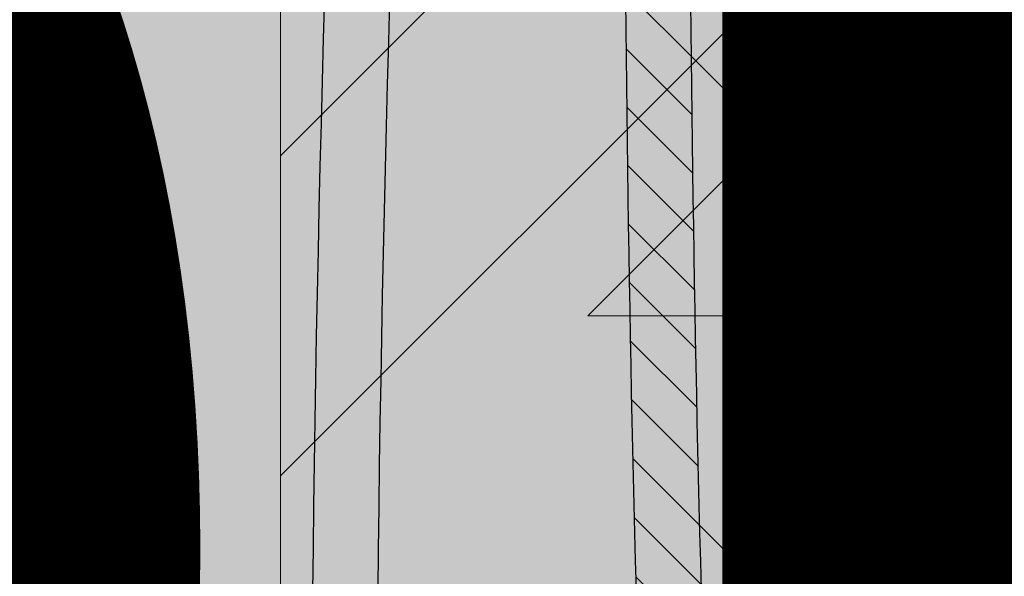
# Model space of a CAD drawing. Units: inches. Extents: x 844 to 2234, y 346 to 1084.
# Tile 76 of 93: x 1998.757 to 2001.166, y 701.365 to 702.727. Entities that reach past the tile are written whole.
import ezdxf

# ---------------------------------------------------------------- set-up
doc = ezdxf.new("R2010")
doc.units = ezdxf.units.IN
doc.header["$MEASUREMENT"] = 0
for name, color, linetype, lineweight in [('A-ANNO-DIMS', 2, 'Continuous', 18), ('furniture', 8, 'Continuous', 18), ('RA-AP-01$0$INT', 35, 'Continuous', 5)]:
    doc.layers.add(name, color=color, linetype=linetype, lineweight=lineweight)
doc.layers.add('RA-AP-01$0$FURN', color=3, linetype='Continuous')
doc.layers.add('RA-AP-01$0$WOOD', color=64, linetype='Continuous')
doc.styles.get("Standard").update_dxf_attribs({"font": 'arial.ttf'})
doc.dimstyles.get("Standard").update_dxf_attribs({"dimtxt": 6, "dimasz": 3, "dimexe": 0.18, "dimexo": 0.0625, "dimgap": 0.09, "dimtad": 0, "dimtih": 1, "dimtoh": 1, "dimdec": 1, "dimzin": 0, "dimdsep": 46, "dimlunit": 3, "dimtxsty": 'Standard', "dimblk": 'ARCHTICK', "dimcen": 0.09, "dimadec": 0, "dimazin": 0, "dimtfac": 1, "dimtdec": 1, "dimtofl": 0, "dimtmove": 0, "dimatfit": 3, "dimfxl": 1, "dimtolj": 1, "dimtzin": 0, "dimarcsym": 0})

# ---------------------------------------------------------------- blocks, each defined once
blk = doc.blocks.new('A$C18D01794')
at = {"layer": 'RA-AP-01$0$INT'}
h = blk.add_hatch(color=256, dxfattribs=at)
h.paths.add_polyline_path([(4.46935, -7.07085), (4.50521, -7.035), (4.50521, -7.10671)])
h.paths.add_polyline_path([(4.45521, -7.085), (4.47692, -7.10671), (4.43349, -7.10671)])
h.paths.add_polyline_path([(4.40521, -7.035), (4.44106, -7.07085), (4.40521, -7.10671)])
h.paths.add_polyline_path([(4.42521, -6.91146), (4.45521, -6.88146), (4.48521, -6.91146), (4.48521, -7.02671), (4.45521, -7.05671), (4.42521, -7.02671)])
h.paths.add_polyline_path([(4.50521, -6.83146), (4.50521, -6.90318), (4.46935, -6.86732)])
h.paths.add_polyline_path([(4.42521, -6.70793), (4.45521, -6.67793), (4.48521, -6.70793), (4.48521, -6.82318), (4.45521, -6.85318), (4.42521, -6.82318)])
h.paths.add_polyline_path([(4.42521, -6.50439), (4.45521, -6.47439), (4.48521, -6.50439), (4.48521, -6.61964), (4.45521, -6.64964), (4.42521, -6.61964)])
h.paths.add_polyline_path([(4.46935, -6.66378), (4.50521, -6.62793), (4.50521, -6.69964)])
h.paths.add_polyline_path([(4.40521, -6.62793), (4.44106, -6.66378), (4.40521, -6.69964)])
h.paths.add_polyline_path([(4.40521, -6.42439), (4.44106, -6.46025), (4.40521, -6.49611)])
h.paths.add_polyline_path([(4.46935, -6.46025), (4.50521, -6.42439), (4.50521, -6.49611)])
h.paths.add_polyline_path([(4.42521, -6.30085), (4.45521, -6.27085), (4.48521, -6.30085), (4.48521, -6.41611), (4.45521, -6.44611), (4.42521, -6.41611)])
h.paths.add_polyline_path([(4.42521, -6.22671), (4.47106, -6.22671), (4.42521, -6.27257)])
h.paths.add_polyline_path([(4.49935, -6.22671), (4.63606, -6.22671), (4.66606, -6.25671), (4.63606, -6.28671), (4.49935, -6.28671), (4.46935, -6.25671)])
h.paths.add_polyline_path([(4.68021, -6.27085), (4.71606, -6.30671), (4.64435, -6.30671)])
h.paths.add_polyline_path([(4.64435, -6.20671), (4.71606, -6.20671), (4.68021, -6.24257)])
h.paths.add_polyline_path([(4.72435, -6.22671), (4.86106, -6.22671), (4.89106, -6.25671), (4.86106, -6.28671), (4.72435, -6.28671), (4.69435, -6.25671)])
h.paths.add_polyline_path([(4.90521, -6.27085), (4.94106, -6.30671), (4.86935, -6.30671)])
h.paths.add_polyline_path([(4.86935, -6.20671), (4.94106, -6.20671), (4.90521, -6.24257)])
h.paths.add_polyline_path([(4.94935, -6.22671), (5.08606, -6.22671), (5.11606, -6.25671), (5.08606, -6.28671), (4.94935, -6.28671), (4.91935, -6.25671)])
h.paths.add_polyline_path([(5.13021, -6.27085), (5.16606, -6.30671), (5.09435, -6.30671)])
h.paths.add_polyline_path([(5.09435, -6.20671), (5.16606, -6.20671), (5.13021, -6.24257)])
h.paths.add_polyline_path([(5.17435, -6.22671), (5.31106, -6.22671), (5.34106, -6.25671), (5.31106, -6.28671), (5.17435, -6.28671), (5.14435, -6.25671)])
h.paths.add_polyline_path([(5.32521, -6.30085), (5.35521, -6.27085), (5.38521, -6.30085), (5.38521, -6.41611), (5.35521, -6.44611), (5.32521, -6.41611)])
h.paths.add_polyline_path([(5.33935, -6.22671), (5.38521, -6.22671), (5.38521, -6.27257)])
h.paths.add_polyline_path([(5.32521, -6.50439), (5.35521, -6.47439), (5.38521, -6.50439), (5.38521, -6.61964), (5.35521, -6.64964), (5.32521, -6.61964)])
h.paths.add_polyline_path([(5.30521, -6.42439), (5.34106, -6.46025), (5.30521, -6.49611)])
h.paths.add_polyline_path([(5.36935, -6.46025), (5.40521, -6.42439), (5.40521, -6.49611)])
h.paths.add_polyline_path([(5.40521, -6.62793), (5.40521, -6.69964), (5.36935, -6.66378)])
h.paths.add_polyline_path([(5.30521, -6.62793), (5.34106, -6.66378), (5.30521, -6.69964)])
h.paths.add_polyline_path([(5.32521, -6.70793), (5.35521, -6.67793), (5.38521, -6.70793), (5.38521, -6.82318), (5.35521, -6.85318), (5.32521, -6.82318)])
h.paths.add_polyline_path([(5.30521, -6.83146), (5.34106, -6.86732), (5.30521, -6.90318)])
h.paths.add_polyline_path([(5.32521, -6.91146), (5.35521, -6.88146), (5.38521, -6.91146), (5.38521, -7.02671), (5.35521, -7.05671), (5.32521, -7.02671)])
h.paths.add_polyline_path([(5.40458, -6.83209, 0.001218), (5.40521, -6.83231), (5.40521, -6.90318), (5.36935, -6.86732)])
h.paths.add_polyline_path([(5.36935, -7.07085), (5.40521, -7.035), (5.40521, -7.10671)])
h.paths.add_polyline_path([(5.35521, -7.085), (5.37692, -7.10671), (5.33349, -7.10671)])
h.paths.add_polyline_path([(5.30521, -7.035), (5.34106, -7.07085), (5.30521, -7.10671)])
for points in [[(4.50521, -6.30671), (5.30521, -6.30671), (5.30521, -7.10671), (5.25521, -7.10671), (5.25521, -6.35671), (4.55521, -6.35671), (4.55521, -7.10671), (4.50521, -7.10671)], [(4.50521, -7.90671), (5.30521, -7.90671), (5.30521, -7.10671), (5.25521, -7.10671), (5.25521, -7.85671), (4.55521, -7.85671), (4.55521, -7.10671), (4.50521, -7.10671)]]:
    blk.add_hatch(color=256, dxfattribs=at).paths.add_polyline_path(points)
h = blk.add_hatch(color=256, dxfattribs=at)
h.paths.add_polyline_path([(4.58592, -6.35671), (4.6142, -6.35671), (4.66885, -6.41136), (4.72349, -6.35671), (4.77177, -6.35671), (4.82642, -6.41136), (4.86278, -6.375), (4.8445, -6.35671), (4.86278, -6.35671), (4.90521, -6.39914), (4.94763, -6.35671), (4.96592, -6.35671), (4.94763, -6.375), (4.98399, -6.41136), (5.03864, -6.35671), (5.08692, -6.35671), (5.14157, -6.41136), (5.19621, -6.35671), (5.2245, -6.35671), (4.90521, -6.676)])
h.paths.add_polyline_path([(4.89521, -6.63772), (4.89521, -6.52843), (4.84056, -6.58307)], flags=16)
h.paths.add_polyline_path([(4.91521, -6.63772), (4.96985, -6.58307), (4.91521, -6.52843)], flags=16)
h.paths.add_polyline_path([(4.82642, -6.56893), (4.88106, -6.51429), (4.77177, -6.51429)], flags=16)
h.paths.add_polyline_path([(4.98399, -6.56893), (5.03864, -6.51429), (4.92935, -6.51429)], flags=16)
h.paths.add_polyline_path([(4.88106, -6.49429), (4.82642, -6.43964), (4.77177, -6.49429)], flags=16)
h.paths.add_polyline_path([(4.92935, -6.49429), (5.03864, -6.49429), (4.98399, -6.43964)], flags=16)
h.paths.add_polyline_path([(4.89521, -6.48014), (4.89521, -6.40742), (4.87692, -6.38914), (4.84056, -6.4255)], flags=16)
h.paths.add_polyline_path([(4.91521, -6.48014), (4.96985, -6.4255), (4.93349, -6.38914), (4.91521, -6.40742)], flags=16)
h.paths.add_polyline_path([(4.75763, -6.48014), (4.81228, -6.4255), (4.75763, -6.37085)], flags=16)
h.paths.add_polyline_path([(4.73763, -6.48014), (4.73763, -6.37085), (4.68299, -6.4255)], flags=16)
h.paths.add_polyline_path([(5.05278, -6.48014), (5.05278, -6.37085), (4.99814, -6.4255)], flags=16)
h.paths.add_polyline_path([(5.07278, -6.48014), (5.12742, -6.4255), (5.07278, -6.37085)], flags=16)
h.paths.add_polyline_path([(4.93592, -6.70671), (5.25521, -6.38742), (5.25521, -6.41571), (5.20056, -6.47035), (5.25521, -6.525), (5.25521, -6.57328), (5.20056, -6.62793), (5.23692, -6.66429), (5.25521, -6.646), (5.25521, -6.66429), (5.21278, -6.70671), (5.25521, -6.74914), (5.25521, -6.76742), (5.23692, -6.74914), (5.20056, -6.7855), (5.25521, -6.84014), (5.25521, -6.88843), (5.20056, -6.94307), (5.25521, -6.99772), (5.25521, -7.026)])
h.paths.add_polyline_path([(5.04299, -6.7855), (5.09763, -6.84014), (5.09763, -6.73085)], flags=16)
h.paths.add_polyline_path([(5.02885, -6.77136), (5.08349, -6.71671), (4.9742, -6.71671)], flags=16)
h.paths.add_polyline_path([(5.11763, -6.84014), (5.17228, -6.7855), (5.11763, -6.73085)], flags=16)
h.paths.add_polyline_path([(5.08349, -6.69671), (5.02885, -6.64207), (4.9742, -6.69671)], flags=16)
h.paths.add_polyline_path([(5.13177, -6.85429), (5.18642, -6.79964), (5.24106, -6.85429)], flags=17)
h.paths.add_polyline_path([(5.13177, -6.71671), (5.18642, -6.77136), (5.22278, -6.735), (5.2045, -6.71671)], flags=16)
h.paths.add_polyline_path([(5.09763, -6.68257), (5.09763, -6.57328), (5.04299, -6.62793)], flags=16)
h.paths.add_polyline_path([(5.13177, -6.87429), (5.24106, -6.87429), (5.18642, -6.92893)], flags=17)
h.paths.add_polyline_path([(5.13177, -6.69671), (5.2045, -6.69671), (5.22278, -6.67843), (5.18642, -6.64207)], flags=16)
h.paths.add_polyline_path([(5.11763, -6.68257), (5.17228, -6.62793), (5.11763, -6.57328)], flags=16)
h.paths.add_polyline_path([(5.18642, -6.61378), (5.24106, -6.55914), (5.13177, -6.55914)], flags=16)
h.paths.add_polyline_path([(5.13177, -6.53914), (5.24106, -6.53914), (5.18642, -6.48449)], flags=16)
h.paths.add_polyline_path([(5.25521, -7.08742), (5.25521, -7.10671), (4.55521, -7.10671), (4.55521, -7.08742), (4.90521, -6.73742)])
h.paths.add_polyline_path([(4.98399, -6.84449), (4.92935, -6.89914), (5.03864, -6.89914)], flags=16)
h.paths.add_polyline_path([(4.96985, -6.83035), (4.91521, -6.77571), (4.91521, -6.885)], flags=16)
h.paths.add_polyline_path([(4.92935, -6.91914), (4.98399, -6.97378), (5.03864, -6.91914)], flags=16)
h.paths.add_polyline_path([(5.05278, -6.93328), (4.99814, -6.98793), (5.05278, -7.04257)], flags=16)
h.paths.add_polyline_path([(5.07278, -6.93328), (5.07278, -7.04257), (5.12742, -6.98793)], flags=16)
h.paths.add_polyline_path([(4.89521, -6.77571), (4.84056, -6.83035), (4.89521, -6.885)], flags=16)
h.paths.add_polyline_path([(4.91521, -6.93328), (4.91521, -7.006), (4.93349, -7.02429), (4.96985, -6.98793)], flags=16)
h.paths.add_polyline_path([(4.88106, -6.89914), (4.82642, -6.84449), (4.77177, -6.89914)], flags=16)
h.paths.add_polyline_path([(4.89521, -6.93328), (4.84056, -6.98793), (4.87692, -7.02429), (4.89521, -7.006)], flags=16)
h.paths.add_polyline_path([(4.98399, -7.00207), (4.94763, -7.03843), (4.96592, -7.05671), (5.03864, -7.05671)], flags=16)
h.paths.add_polyline_path([(4.88106, -6.91914), (4.77177, -6.91914), (4.82642, -6.97378)], flags=16)
h.paths.add_polyline_path([(4.90521, -7.01429), (4.86278, -7.05671), (4.94763, -7.05671)], flags=16)
h.paths.add_polyline_path([(5.14157, -7.00207), (5.08692, -7.05671), (5.19621, -7.05671)], flags=16)
h.paths.add_polyline_path([(4.82642, -7.00207), (4.77177, -7.05671), (4.8445, -7.05671), (4.86278, -7.03843)], flags=16)
h.paths.add_polyline_path([(4.81228, -6.98793), (4.75763, -6.93328), (4.75763, -7.04257)], flags=16)
h.paths.add_polyline_path([(4.73763, -6.93328), (4.68299, -6.98793), (4.73763, -7.04257)], flags=16)
h.paths.add_polyline_path([(4.72349, -7.05671), (4.66885, -7.00207), (4.6142, -7.05671)], flags=16)
h.paths.add_polyline_path([(4.59763, -6.70671), (4.55521, -6.66429), (4.55521, -6.646), (4.57349, -6.66429), (4.60985, -6.62793), (4.55521, -6.57328), (4.55521, -6.525), (4.60985, -6.47035), (4.55521, -6.41571), (4.55521, -6.38742), (4.8745, -6.70671), (4.55521, -7.026), (4.55521, -6.99772), (4.60985, -6.94307), (4.55521, -6.88843), (4.55521, -6.84014), (4.60985, -6.7855), (4.57349, -6.74914), (4.55521, -6.76742), (4.55521, -6.74914)])
h.paths.add_polyline_path([(4.71278, -6.73085), (4.71278, -6.84014), (4.76742, -6.7855)], flags=16)
h.paths.add_polyline_path([(4.72692, -6.71671), (4.78157, -6.77136), (4.83621, -6.71671)], flags=16)
h.paths.add_polyline_path([(4.69278, -6.73085), (4.63814, -6.7855), (4.69278, -6.84014)], flags=16)
h.paths.add_polyline_path([(4.72692, -6.69671), (4.83621, -6.69671), (4.78157, -6.64207)], flags=16)
h.paths.add_polyline_path([(4.67864, -6.71671), (4.60592, -6.71671), (4.58763, -6.735), (4.62399, -6.77136)], flags=16)
h.paths.add_polyline_path([(4.71278, -6.68257), (4.76742, -6.62793), (4.71278, -6.57328)], flags=16)
h.paths.add_polyline_path([(4.67864, -6.69671), (4.62399, -6.64207), (4.58763, -6.67843), (4.60592, -6.69671)], flags=16)
h.paths.add_polyline_path([(4.69278, -6.68257), (4.69278, -6.57328), (4.63814, -6.62793)], flags=16)
h.paths.add_polyline_path([(4.62399, -6.79964), (4.67864, -6.85429), (4.56935, -6.85429)], flags=17)
h.paths.add_polyline_path([(4.62399, -6.61378), (4.67864, -6.55914), (4.56935, -6.55914)], flags=16)
h.paths.add_polyline_path([(4.67864, -6.87429), (4.62399, -6.92893), (4.56935, -6.87429)], flags=17)
h.paths.add_polyline_path([(4.67864, -6.53914), (4.62399, -6.48449), (4.56935, -6.53914)], flags=16)
h = blk.add_hatch(color=256, dxfattribs=at)
h.paths.add_polyline_path([(4.50521, -7.5855), (4.46935, -7.54964), (4.50521, -7.51378), (4.50521, -7.38196), (4.46935, -7.34611), (4.50521, -7.31025), (4.50521, -7.17843), (4.46935, -7.14257), (4.50521, -7.10671), (4.47692, -7.10671), (4.45521, -7.12843), (4.43349, -7.10671), (4.40521, -7.10671), (4.44106, -7.14257), (4.40521, -7.17843), (4.40521, -7.31025), (4.44106, -7.34611), (4.40521, -7.38196), (4.40521, -7.51378), (4.44106, -7.54964), (4.40521, -7.5855), (4.40521, -7.71732), (4.44106, -7.75318), (4.40521, -7.78903), (4.40521, -8.00671), (4.64435, -8.00671), (4.68021, -7.97085), (4.71606, -8.00671), (4.86935, -8.00671), (4.90521, -7.97085), (4.94106, -8.00671), (5.09435, -8.00671), (5.13021, -7.97085), (5.16606, -8.00671), (5.40521, -8.00671), (5.40521, -7.78903), (5.36935, -7.75318), (5.40521, -7.71732), (5.40521, -7.5855), (5.36935, -7.54964), (5.40521, -7.51378), (5.40521, -7.38196), (5.36935, -7.34611), (5.40521, -7.31025), (5.40521, -7.17843), (5.36935, -7.14257), (5.40521, -7.10671), (5.37692, -7.10671), (5.35521, -7.12843), (5.33349, -7.10671), (5.30521, -7.10671), (5.34106, -7.14257), (5.30521, -7.17843), (5.30521, -7.31025), (5.34106, -7.34611), (5.30521, -7.38196), (5.30521, -7.51378), (5.34106, -7.54964), (5.30521, -7.5855), (5.30521, -7.71732), (5.34106, -7.75318), (5.30521, -7.78903), (5.30521, -7.90671), (5.16606, -7.90671), (5.13021, -7.94257), (5.09435, -7.90671), (4.94106, -7.90671), (4.90521, -7.94257), (4.86935, -7.90671), (4.71606, -7.90671), (4.68021, -7.94257), (4.64435, -7.90671), (4.50521, -7.90671), (4.50521, -7.78903), (4.46935, -7.75318), (4.50521, -7.71732)])
h.paths.add_polyline_path([(4.48521, -7.70903), (4.45521, -7.73903), (4.42521, -7.70903), (4.42521, -7.59378), (4.45521, -7.56378), (4.48521, -7.59378)], flags=16)
h.paths.add_polyline_path([(4.45521, -7.76732), (4.48521, -7.79732), (4.48521, -7.91257), (4.45521, -7.94257), (4.42521, -7.91257), (4.42521, -7.79732)], flags=16)
h.paths.add_polyline_path([(4.45521, -7.5355), (4.42521, -7.5055), (4.42521, -7.39025), (4.45521, -7.36025), (4.48521, -7.39025), (4.48521, -7.5055)], flags=16)
h.paths.add_polyline_path([(4.49935, -7.92671), (4.63606, -7.92671), (4.66606, -7.95671), (4.63606, -7.98671), (4.49935, -7.98671), (4.46935, -7.95671)], flags=16)
h.paths.add_polyline_path([(4.42521, -7.94085), (4.47106, -7.98671), (4.42521, -7.98671)], flags=16)
h.paths.add_polyline_path([(4.45521, -7.33196), (4.42521, -7.30196), (4.42521, -7.18671), (4.45521, -7.15671), (4.48521, -7.18671), (4.48521, -7.30196)], flags=16)
h.paths.add_polyline_path([(4.72435, -7.92671), (4.86106, -7.92671), (4.89106, -7.95671), (4.86106, -7.98671), (4.72435, -7.98671), (4.69435, -7.95671)], flags=16)
h.paths.add_polyline_path([(4.91935, -7.95671), (4.94935, -7.92671), (5.08606, -7.92671), (5.11606, -7.95671), (5.08606, -7.98671), (4.94935, -7.98671)], flags=16)
h.paths.add_polyline_path([(5.14435, -7.95671), (5.17435, -7.92671), (5.31106, -7.92671), (5.34106, -7.95671), (5.31106, -7.98671), (5.17435, -7.98671)], flags=16)
h.paths.add_polyline_path([(5.32521, -7.59378), (5.35521, -7.56378), (5.38521, -7.59378), (5.38521, -7.70903), (5.35521, -7.73903), (5.32521, -7.70903)], flags=16)
h.paths.add_polyline_path([(5.32521, -7.79732), (5.35521, -7.76732), (5.38521, -7.79732), (5.38521, -7.91257), (5.35521, -7.94257), (5.32521, -7.91257)], flags=16)
h.paths.add_polyline_path([(5.32521, -7.5055), (5.32521, -7.39025), (5.35521, -7.36025), (5.38521, -7.39025), (5.38521, -7.5055), (5.35521, -7.5355)], flags=16)
h.paths.add_polyline_path([(5.32521, -7.30196), (5.32521, -7.18671), (5.35521, -7.15671), (5.38521, -7.18671), (5.38521, -7.30196), (5.35521, -7.33196)], flags=16)
h.paths.add_polyline_path([(5.33935, -7.98671), (5.38521, -7.94085), (5.38521, -7.98671)], flags=16)
h = blk.add_hatch(color=256, dxfattribs=at)
h.paths.add_polyline_path([(4.46935, -7.14257), (4.50521, -7.17843), (4.50521, -7.10671)])
h.paths.add_polyline_path([(4.45521, -7.12843), (4.47692, -7.10671), (4.43349, -7.10671)])
h.paths.add_polyline_path([(4.40521, -7.17843), (4.44106, -7.14257), (4.40521, -7.10671)])
h.paths.add_polyline_path([(4.42521, -7.30196), (4.45521, -7.33196), (4.48521, -7.30196), (4.48521, -7.18671), (4.45521, -7.15671), (4.42521, -7.18671)])
h.paths.add_polyline_path([(4.50521, -7.38196), (4.50521, -7.31025), (4.46935, -7.34611)])
h.paths.add_polyline_path([(4.42521, -7.5055), (4.45521, -7.5355), (4.48521, -7.5055), (4.48521, -7.39025), (4.45521, -7.36025), (4.42521, -7.39025)])
h.paths.add_polyline_path([(4.42521, -7.70903), (4.45521, -7.73903), (4.48521, -7.70903), (4.48521, -7.59378), (4.45521, -7.56378), (4.42521, -7.59378)])
h.paths.add_polyline_path([(4.46935, -7.54964), (4.50521, -7.5855), (4.50521, -7.51378)])
h.paths.add_polyline_path([(4.40521, -7.5855), (4.44106, -7.54964), (4.40521, -7.51378)])
h.paths.add_polyline_path([(4.40521, -7.78903), (4.44106, -7.75318), (4.40521, -7.71732)])
h.paths.add_polyline_path([(4.46935, -7.75318), (4.50521, -7.78903), (4.50521, -7.71732)])
h.paths.add_polyline_path([(4.42521, -7.91257), (4.45521, -7.94257), (4.48521, -7.91257), (4.48521, -7.79732), (4.45521, -7.76732), (4.42521, -7.79732)])
h.paths.add_polyline_path([(4.42521, -7.98671), (4.47106, -7.98671), (4.42521, -7.94085)])
h.paths.add_polyline_path([(4.49935, -7.98671), (4.63606, -7.98671), (4.66606, -7.95671), (4.63606, -7.92671), (4.49935, -7.92671), (4.46935, -7.95671)])
h.paths.add_polyline_path([(4.68021, -7.94257), (4.71606, -7.90671), (4.64435, -7.90671)])
h.paths.add_polyline_path([(4.64435, -8.00671), (4.71606, -8.00671), (4.68021, -7.97085)])
h.paths.add_polyline_path([(4.72435, -7.98671), (4.86106, -7.98671), (4.89106, -7.95671), (4.86106, -7.92671), (4.72435, -7.92671), (4.69435, -7.95671)])
h.paths.add_polyline_path([(4.90521, -7.94257), (4.94106, -7.90671), (4.86935, -7.90671)])
h.paths.add_polyline_path([(4.86935, -8.00671), (4.94106, -8.00671), (4.90521, -7.97085)])
h.paths.add_polyline_path([(4.94935, -7.98671), (5.08606, -7.98671), (5.11606, -7.95671), (5.08606, -7.92671), (4.94935, -7.92671), (4.91935, -7.95671)])
h.paths.add_polyline_path([(5.13021, -7.94257), (5.16606, -7.90671), (5.09435, -7.90671)])
h.paths.add_polyline_path([(5.09435, -8.00671), (5.16606, -8.00671), (5.13021, -7.97085)])
h.paths.add_polyline_path([(5.17435, -7.98671), (5.31106, -7.98671), (5.34106, -7.95671), (5.31106, -7.92671), (5.17435, -7.92671), (5.14435, -7.95671)])
h.paths.add_polyline_path([(5.32521, -7.91257), (5.35521, -7.94257), (5.38521, -7.91257), (5.38521, -7.79732), (5.35521, -7.76732), (5.32521, -7.79732)])
h.paths.add_polyline_path([(5.33935, -7.98671), (5.38521, -7.98671), (5.38521, -7.94085)])
h.paths.add_polyline_path([(5.32521, -7.70903), (5.35521, -7.73903), (5.38521, -7.70903), (5.38521, -7.59378), (5.35521, -7.56378), (5.32521, -7.59378)])
h.paths.add_polyline_path([(5.30521, -7.78903), (5.34106, -7.75318), (5.30521, -7.71732)])
h.paths.add_polyline_path([(5.36935, -7.75318), (5.40521, -7.78903), (5.40521, -7.71732)])
h.paths.add_polyline_path([(5.40521, -7.5855), (5.40521, -7.51378), (5.36935, -7.54964)])
h.paths.add_polyline_path([(5.30521, -7.5855), (5.34106, -7.54964), (5.30521, -7.51378)])
h.paths.add_polyline_path([(5.32521, -7.5055), (5.35521, -7.5355), (5.38521, -7.5055), (5.38521, -7.39025), (5.35521, -7.36025), (5.32521, -7.39025)])
h.paths.add_polyline_path([(5.30521, -7.38196), (5.34106, -7.34611), (5.30521, -7.31025)])
h.paths.add_polyline_path([(5.32521, -7.30196), (5.35521, -7.33196), (5.38521, -7.30196), (5.38521, -7.18671), (5.35521, -7.15671), (5.32521, -7.18671)])
h.paths.add_polyline_path([(5.40458, -7.38134, -0.001218), (5.40521, -7.38111), (5.40521, -7.31025), (5.36935, -7.34611)])
h.paths.add_polyline_path([(5.36935, -7.14257), (5.40521, -7.17843), (5.40521, -7.10671)])
h.paths.add_polyline_path([(5.35521, -7.12843), (5.37692, -7.10671), (5.33349, -7.10671)])
h.paths.add_polyline_path([(5.30521, -7.17843), (5.34106, -7.14257), (5.30521, -7.10671)])
h = blk.add_hatch(color=256, dxfattribs=at)
h.paths.add_polyline_path([(4.58592, -7.85671), (4.6142, -7.85671), (4.66885, -7.80207), (4.72349, -7.85671), (4.77177, -7.85671), (4.82642, -7.80207), (4.86278, -7.83843), (4.8445, -7.85671), (4.86278, -7.85671), (4.90521, -7.81429), (4.94763, -7.85671), (4.96592, -7.85671), (4.94763, -7.83843), (4.98399, -7.80207), (5.03864, -7.85671), (5.08692, -7.85671), (5.14157, -7.80207), (5.19621, -7.85671), (5.2245, -7.85671), (4.90521, -7.53742)])
h.paths.add_polyline_path([(4.89521, -7.57571), (4.89521, -7.685), (4.84056, -7.63035)], flags=16)
h.paths.add_polyline_path([(4.91521, -7.57571), (4.96985, -7.63035), (4.91521, -7.685)], flags=16)
h.paths.add_polyline_path([(4.82642, -7.64449), (4.88106, -7.69914), (4.77177, -7.69914)], flags=16)
h.paths.add_polyline_path([(4.98399, -7.64449), (5.03864, -7.69914), (4.92935, -7.69914)], flags=16)
h.paths.add_polyline_path([(4.88106, -7.71914), (4.82642, -7.77378), (4.77177, -7.71914)], flags=16)
h.paths.add_polyline_path([(4.92935, -7.71914), (5.03864, -7.71914), (4.98399, -7.77378)], flags=16)
h.paths.add_polyline_path([(4.89521, -7.73328), (4.89521, -7.806), (4.87692, -7.82429), (4.84056, -7.78793)], flags=16)
h.paths.add_polyline_path([(4.91521, -7.73328), (4.96985, -7.78793), (4.93349, -7.82429), (4.91521, -7.806)], flags=16)
h.paths.add_polyline_path([(4.75763, -7.73328), (4.81228, -7.78793), (4.75763, -7.84257)], flags=16)
h.paths.add_polyline_path([(4.73763, -7.73328), (4.73763, -7.84257), (4.68299, -7.78793)], flags=16)
h.paths.add_polyline_path([(5.05278, -7.73328), (5.05278, -7.84257), (4.99814, -7.78793)], flags=16)
h.paths.add_polyline_path([(5.07278, -7.73328), (5.12742, -7.78793), (5.07278, -7.84257)], flags=16)
h.paths.add_polyline_path([(4.93592, -7.50671), (5.25521, -7.826), (5.25521, -7.79772), (5.20056, -7.74307), (5.25521, -7.68843), (5.25521, -7.64014), (5.20056, -7.5855), (5.23692, -7.54914), (5.25521, -7.56742), (5.25521, -7.54914), (5.21278, -7.50671), (5.25521, -7.46429), (5.25521, -7.446), (5.23692, -7.46429), (5.20056, -7.42793), (5.25521, -7.37328), (5.25521, -7.325), (5.20056, -7.27035), (5.25521, -7.21571), (5.25521, -7.18742)])
h.paths.add_polyline_path([(5.04299, -7.42793), (5.09763, -7.37328), (5.09763, -7.48257)], flags=16)
h.paths.add_polyline_path([(5.02885, -7.44207), (5.08349, -7.49671), (4.9742, -7.49671)], flags=16)
h.paths.add_polyline_path([(5.11763, -7.37328), (5.17228, -7.42793), (5.11763, -7.48257)], flags=16)
h.paths.add_polyline_path([(5.08349, -7.51671), (5.02885, -7.57136), (4.9742, -7.51671)], flags=16)
h.paths.add_polyline_path([(5.13177, -7.35914), (5.18642, -7.41378), (5.24106, -7.35914)], flags=17)
h.paths.add_polyline_path([(5.13177, -7.49671), (5.18642, -7.44207), (5.22278, -7.47843), (5.2045, -7.49671)], flags=16)
h.paths.add_polyline_path([(5.09763, -7.53085), (5.09763, -7.64014), (5.04299, -7.5855)], flags=16)
h.paths.add_polyline_path([(5.13177, -7.33914), (5.24106, -7.33914), (5.18642, -7.28449)], flags=17)
h.paths.add_polyline_path([(5.13177, -7.51671), (5.2045, -7.51671), (5.22278, -7.535), (5.18642, -7.57136)], flags=16)
h.paths.add_polyline_path([(5.11763, -7.53085), (5.17228, -7.5855), (5.11763, -7.64014)], flags=16)
h.paths.add_polyline_path([(5.18642, -7.59964), (5.24106, -7.65429), (5.13177, -7.65429)], flags=16)
h.paths.add_polyline_path([(5.13177, -7.67429), (5.24106, -7.67429), (5.18642, -7.72893)], flags=16)
h.paths.add_polyline_path([(5.25521, -7.126), (5.25521, -7.10671), (4.55521, -7.10671), (4.55521, -7.126), (4.90521, -7.476)])
h.paths.add_polyline_path([(4.98399, -7.36893), (4.92935, -7.31429), (5.03864, -7.31429)], flags=16)
h.paths.add_polyline_path([(4.96985, -7.38307), (4.91521, -7.43772), (4.91521, -7.32843)], flags=16)
h.paths.add_polyline_path([(4.92935, -7.29429), (4.98399, -7.23964), (5.03864, -7.29429)], flags=16)
h.paths.add_polyline_path([(5.05278, -7.28014), (4.99814, -7.2255), (5.05278, -7.17085)], flags=16)
h.paths.add_polyline_path([(5.07278, -7.28014), (5.07278, -7.17085), (5.12742, -7.2255)], flags=16)
h.paths.add_polyline_path([(4.89521, -7.43772), (4.84056, -7.38307), (4.89521, -7.32843)], flags=16)
h.paths.add_polyline_path([(4.91521, -7.28014), (4.91521, -7.20742), (4.93349, -7.18914), (4.96985, -7.2255)], flags=16)
h.paths.add_polyline_path([(4.88106, -7.31429), (4.82642, -7.36893), (4.77177, -7.31429)], flags=16)
h.paths.add_polyline_path([(4.89521, -7.28014), (4.84056, -7.2255), (4.87692, -7.18914), (4.89521, -7.20742)], flags=16)
h.paths.add_polyline_path([(4.98399, -7.21136), (4.94763, -7.175), (4.96592, -7.15671), (5.03864, -7.15671)], flags=16)
h.paths.add_polyline_path([(4.88106, -7.29429), (4.77177, -7.29429), (4.82642, -7.23964)], flags=16)
h.paths.add_polyline_path([(4.90521, -7.19914), (4.86278, -7.15671), (4.94763, -7.15671)], flags=16)
h.paths.add_polyline_path([(5.14157, -7.21136), (5.08692, -7.15671), (5.19621, -7.15671)], flags=16)
h.paths.add_polyline_path([(4.82642, -7.21136), (4.77177, -7.15671), (4.8445, -7.15671), (4.86278, -7.175)], flags=16)
h.paths.add_polyline_path([(4.81228, -7.2255), (4.75763, -7.28014), (4.75763, -7.17085)], flags=16)
h.paths.add_polyline_path([(4.73763, -7.28014), (4.68299, -7.2255), (4.73763, -7.17085)], flags=16)
h.paths.add_polyline_path([(4.72349, -7.15671), (4.66885, -7.21136), (4.6142, -7.15671)], flags=16)
h.paths.add_polyline_path([(4.59763, -7.50671), (4.55521, -7.54914), (4.55521, -7.56742), (4.57349, -7.54914), (4.60985, -7.5855), (4.55521, -7.64014), (4.55521, -7.68843), (4.60985, -7.74307), (4.55521, -7.79772), (4.55521, -7.826), (4.8745, -7.50671), (4.55521, -7.18742), (4.55521, -7.21571), (4.60985, -7.27035), (4.55521, -7.325), (4.55521, -7.37328), (4.60985, -7.42793), (4.57349, -7.46429), (4.55521, -7.446), (4.55521, -7.46429)])
h.paths.add_polyline_path([(4.71278, -7.48257), (4.71278, -7.37328), (4.76742, -7.42793)], flags=16)
h.paths.add_polyline_path([(4.72692, -7.49671), (4.78157, -7.44207), (4.83621, -7.49671)], flags=16)
h.paths.add_polyline_path([(4.69278, -7.48257), (4.63814, -7.42793), (4.69278, -7.37328)], flags=16)
h.paths.add_polyline_path([(4.72692, -7.51671), (4.83621, -7.51671), (4.78157, -7.57136)], flags=16)
h.paths.add_polyline_path([(4.67864, -7.49671), (4.60592, -7.49671), (4.58763, -7.47843), (4.62399, -7.44207)], flags=16)
h.paths.add_polyline_path([(4.71278, -7.53085), (4.76742, -7.5855), (4.71278, -7.64014)], flags=16)
h.paths.add_polyline_path([(4.67864, -7.51671), (4.62399, -7.57136), (4.58763, -7.535), (4.60592, -7.51671)], flags=16)
h.paths.add_polyline_path([(4.69278, -7.53085), (4.69278, -7.64014), (4.63814, -7.5855)], flags=16)
h.paths.add_polyline_path([(4.62399, -7.41378), (4.67864, -7.35914), (4.56935, -7.35914)], flags=17)
h.paths.add_polyline_path([(4.62399, -7.59964), (4.67864, -7.65429), (4.56935, -7.65429)], flags=16)
h.paths.add_polyline_path([(4.67864, -7.33914), (4.62399, -7.28449), (4.56935, -7.33914)], flags=17)
h.paths.add_polyline_path([(4.67864, -7.67429), (4.62399, -7.72893), (4.56935, -7.67429)], flags=16)
h = blk.add_hatch(color=256, dxfattribs=at)
h.paths.add_polyline_path([(4.90521, -7.53742), (4.8745, -7.50671), (4.55521, -7.826), (4.55521, -7.85671), (4.58592, -7.85671)])
h.paths.add_polyline_path([(4.93592, -7.50671), (4.90521, -7.53742), (5.2245, -7.85671), (5.25521, -7.85671), (5.25521, -7.826)])
h.paths.add_polyline_path([(5.25521, -7.18742), (5.25521, -7.126), (4.90521, -7.476), (4.93592, -7.50671)])
h.paths.add_polyline_path([(4.8745, -7.50671), (4.90521, -7.476), (4.55521, -7.126), (4.55521, -7.18742)])
h = blk.add_hatch(color=256, dxfattribs=at)
h.paths.add_polyline_path([(4.89521, -7.32843), (4.84056, -7.38307), (4.89521, -7.43772)])
h.paths.add_polyline_path([(4.91521, -7.43772), (4.96985, -7.38307), (4.91521, -7.32843)])
h.paths.add_polyline_path([(4.92935, -7.31429), (4.98399, -7.36893), (5.03864, -7.31429)])
h.paths.add_polyline_path([(5.03864, -7.29429), (4.98399, -7.23964), (4.92935, -7.29429)])
h.paths.add_polyline_path([(4.96985, -7.2255), (4.93349, -7.18914), (4.91521, -7.20742), (4.91521, -7.28014)])
h.paths.add_polyline_path([(4.96592, -7.15671), (4.94763, -7.175), (4.98399, -7.21136), (5.03864, -7.15671)])
h.paths.add_polyline_path([(4.99814, -7.2255), (5.05278, -7.28014), (5.05278, -7.17085)])
h.paths.add_polyline_path([(5.07278, -7.28014), (5.12742, -7.2255), (5.07278, -7.17085)])
h.paths.add_polyline_path([(5.19621, -7.15671), (5.08692, -7.15671), (5.14157, -7.21136)])
h.paths.add_polyline_path([(4.86278, -7.15671), (4.90521, -7.19914), (4.94763, -7.15671)])
h.paths.add_polyline_path([(4.89521, -7.28014), (4.89521, -7.20742), (4.87692, -7.18914), (4.84056, -7.2255)])
h.paths.add_polyline_path([(4.82642, -7.23964), (4.77177, -7.29429), (4.88106, -7.29429)])
h.paths.add_polyline_path([(4.77177, -7.31429), (4.82642, -7.36893), (4.88106, -7.31429)])
h.paths.add_polyline_path([(4.75763, -7.28014), (4.81228, -7.2255), (4.75763, -7.17085)])
h.paths.add_polyline_path([(4.86278, -7.175), (4.8445, -7.15671), (4.77177, -7.15671), (4.82642, -7.21136)])
h.paths.add_polyline_path([(4.68299, -7.2255), (4.73763, -7.28014), (4.73763, -7.17085)])
h.paths.add_polyline_path([(4.72349, -7.15671), (4.6142, -7.15671), (4.66885, -7.21136)])
for p, q in [((5.25521, -7.10671), (5.25521, -6.35671)), ((5.25521, -7.10671), (5.25521, -7.85671)), ((4.90521, -7.476), (5.25521, -7.126)), ((5.08692, -7.15671), (5.19621, -7.15671)), ((5.08692, -7.15671), (5.14157, -7.21136)), ((5.19621, -7.15671), (5.14157, -7.21136)), ((4.93592, -7.50671), (5.25521, -7.18742))]:
    blk.add_line(p, q, dxfattribs=at)
for points in [[(5.30521, -7.10671), (5.30521, -6.30671), (4.50521, -6.30671), (4.50521, -7.10671)], [(5.30521, -7.10671), (5.30521, -7.90671), (4.50521, -7.90671), (4.50521, -7.10671)]]:
    blk.add_lwpolyline(points, dxfattribs=at)
blk = doc.blocks.new('A$C32926AE1')
at = {"layer": 'RA-AP-01$0$WOOD'}
h = blk.add_hatch(color=256, dxfattribs=at)
h.dxf.hatch_style = 1
h.paths.add_polyline_path([(5.15743, 4.57348, -0.100949), (5.1554, 4.59337, -0.184266), (5.17225, 4.6388, 0.205661), (5.17956, 4.66132, 0.361434), (5.13435, 4.70652, 0.205661), (5.11183, 4.69921, -0.184266), (5.0664, 4.68237, -0.105531), (5.04566, 4.68467, 0.156764), (4.76389, 4.68467, -0.105531), (4.74314, 4.68237, -0.184266), (4.69771, 4.69921, 0.205661), (4.67519, 4.70652, 0.361434), (4.62998, 4.66132, 0.205661), (4.63729, 4.6388, -0.184266), (4.65414, 4.59337, -0.100949), (4.65211, 4.57348, 0.02141), (4.62975, 4.15671, 0.02141), (4.65211, 3.73994, -0.100949), (4.65414, 3.72006, -0.184266), (4.63729, 3.67463, 0.205661), (4.62998, 3.65211, 0.361434), (4.67519, 3.6069, 0.205661), (4.69771, 3.61421, -0.184266), (4.74314, 3.63106, -0.105531), (4.76389, 3.62875, 0.156764), (5.04566, 3.62875, -0.105531), (5.0664, 3.63106, -0.184266), (5.11183, 3.61421, 0.205661), (5.13435, 3.6069, 0.361434), (5.17956, 3.65211, 0.205661), (5.17225, 3.67463, -0.184266), (5.1554, 3.72006, -0.100949), (5.15743, 3.73994, 0.02141), (5.17979, 4.15671, 0.02141)])
h.paths.add_polyline_path([(4.63975, 4.15671, 0.021354), (4.66197, 3.74189, -0.094076), (4.66414, 3.71961, -0.182482), (4.64481, 3.66804, 0.205661), (4.63994, 3.65302, 0.361434), (4.67611, 3.61686, 0.205661), (4.69112, 3.62173, -0.182482), (4.7427, 3.64106, -0.102989), (4.76699, 3.63826, 0.156709), (5.04255, 3.63826, -0.102989), (5.06685, 3.64106, -0.182482), (5.11842, 3.62173, 0.205661), (5.13344, 3.61686, 0.361434), (5.1696, 3.65302, 0.205661), (5.16473, 3.66804, -0.182482), (5.1454, 3.71961, -0.094076), (5.14757, 3.74189, 0.021354), (5.16979, 4.15671, 0.021354), (5.14757, 4.57154, -0.094076), (5.1454, 4.59381, -0.182482), (5.16473, 4.64539, 0.205661), (5.1696, 4.6604, 0.361434), (5.13344, 4.69657, 0.205661), (5.11842, 4.69169, -0.182482), (5.06685, 4.67236, -0.102989), (5.04255, 4.67517, 0.156709), (4.76699, 4.67517, -0.102989), (4.7427, 4.67236, -0.182482), (4.69112, 4.69169, 0.205661), (4.67611, 4.69657, 0.361434), (4.63994, 4.6604, 0.205661), (4.64481, 4.64539, -0.182482), (4.66414, 4.59381, -0.094076), (4.66197, 4.57154, 0.021354)], flags=16)
h.paths.add_polyline_path([(5.12979, 4.43217, -0.014166), (5.13015, 4.15693, -0.014166), (5.12979, 3.88169, -0.078525), (5.1098, 3.75514, 0.094597), (5.10541, 3.7179, 0.104317), (5.11607, 3.67039, 0.104317), (5.06856, 3.68105, 0.094597), (5.03132, 3.67666, -0.158024), (4.77823, 3.67666, 0.094597), (4.74098, 3.68105, 0.104317), (4.69347, 3.67039, 0.104317), (4.70413, 3.7179, 0.094597), (4.69975, 3.75514, -0.078525), (4.67975, 3.88169, -0.014166), (4.67939, 4.15693, -0.014166), (4.67975, 4.43217, -0.078525), (4.69975, 4.55871, 0.094597), (4.70413, 4.59596, 0.104317), (4.69347, 4.64347, 0.104317), (4.74098, 4.6328, 0.094597), (4.77823, 4.63719, -0.158024), (5.03132, 4.63719, 0.094597), (5.06856, 4.6328, 0.104317), (5.11607, 4.64347, 0.104317), (5.10541, 4.59596, 0.094597), (5.1098, 4.55871, -0.078525)], flags=0)
h.paths.add_polyline_path([(5.11979, 4.43226, -0.0142), (5.12016, 4.15693, -0.0142), (5.11979, 3.8816, -0.078489), (5.10027, 3.75819, 0.094014), (5.09541, 3.71748, 0.060627), (5.09962, 3.68684, 0.060627), (5.06898, 3.69105, 0.094014), (5.02827, 3.68619, -0.158071), (4.78127, 3.68619, 0.094014), (4.74056, 3.69105, 0.060627), (4.70993, 3.68684, 0.060627), (4.71413, 3.71748, 0.094014), (4.70927, 3.75819, -0.078489), (4.68975, 3.8816, -0.0142), (4.68939, 4.15693, -0.0142), (4.68975, 4.43226, -0.078489), (4.70927, 4.55566, 0.094014), (4.71413, 4.59638, 0.060627), (4.70993, 4.62701, 0.060627), (4.74056, 4.62281, 0.094014), (4.78127, 4.62767, -0.158071), (5.02827, 4.62767, 0.094014), (5.06898, 4.62281, 0.060627), (5.09962, 4.62701, 0.060627), (5.09541, 4.59638, 0.094014), (5.10027, 4.55566, -0.078489)], flags=0)
h.paths.add_polyline_path([(5.06979, 4.43022, -0.014242), (5.07017, 4.15693, -0.014242), (5.06979, 3.88364, -0.080061), (5.05266, 3.77346, 0.052642), (5.04591, 3.74055, 0.052642), (5.013, 3.7338, -0.158303), (4.79655, 3.7338, 0.052642), (4.76363, 3.74055, 0.052642), (4.75688, 3.77346, -0.080061), (4.73975, 3.88364, -0.014242), (4.73937, 4.15693, -0.014242), (4.73975, 4.43022, -0.080061), (4.75688, 4.54039, 0.052642), (4.76363, 4.5733, 0.052642), (4.79655, 4.58006, -0.158303), (5.013, 4.58006, 0.052642), (5.04591, 4.5733, 0.052642), (5.05266, 4.54039, -0.080061)], flags=0)
h.paths.add_polyline_path([(5.04979, 4.43038, -0.01431), (5.05018, 4.15693, -0.01431), (5.04979, 3.88347, -0.080069), (5.03362, 3.77958, 0.030626), (5.02824, 3.75822, 0.030626), (5.00688, 3.75284, -0.158398), (4.80266, 3.75284, 0.030626), (4.7813, 3.75822, 0.030626), (4.77592, 3.77958, -0.080069), (4.75975, 3.88347, -0.01431), (4.75936, 4.15693, -0.01431), (4.75975, 4.43038, -0.080069), (4.77592, 4.53427, 0.030626), (4.7813, 4.55564, 0.030626), (4.80266, 4.56102, -0.158398), (5.00688, 4.56102, 0.030626), (5.02824, 4.55564, 0.030626), (5.03362, 4.53427, -0.080069)], flags=0)
h.paths.add_polyline_path([(4.99977, 4.42817, -0.014344), (5.0002, 4.15693, -0.014344), (4.99977, 3.88568, -0.078464), (4.98736, 3.7991, -0.150605), (4.82219, 3.7991, -0.078464), (4.80978, 3.88568, -0.014344), (4.80934, 4.15693, -0.014344), (4.80978, 4.42817, -0.078464), (4.82219, 4.51475, -0.150605), (4.98736, 4.51475, -0.078464)], flags=0)
h.paths.add_polyline_path([(4.97976, 4.42764, -0.014377), (4.98021, 4.15693, -0.014377), (4.97976, 3.88621, -0.068924), (4.97118, 3.81528, -0.129665), (4.83836, 3.81528, -0.068924), (4.82979, 3.88621, -0.014377), (4.82934, 4.15693, -0.014377), (4.82979, 4.42764, -0.068924), (4.83836, 4.49858, -0.129665), (4.97118, 4.49858, -0.068924)], flags=0)
h = blk.add_hatch(color=256, dxfattribs=at)
h.dxf.hatch_style = 1
h.paths.add_polyline_path([(5.1454, 4.59381, -0.182482), (5.16473, 4.64539, 0.205661), (5.1696, 4.6604, 0.361434), (5.13344, 4.69657, 0.205661), (5.11842, 4.69169, -0.182482), (5.06685, 4.67236, -0.102989), (5.04255, 4.67517, 0.156709), (4.76699, 4.67517, -0.102989), (4.7427, 4.67236, -0.182482), (4.69112, 4.69169, 0.205661), (4.67611, 4.69657, 0.361434), (4.63994, 4.6604, 0.205661), (4.64481, 4.64539, -0.182482), (4.66414, 4.59381, -0.094076), (4.66197, 4.57154, 0.021354), (4.63975, 4.15671, 0.021354), (4.66197, 3.74189, -0.094076), (4.66414, 3.71961, -0.182482), (4.64481, 3.66804, 0.205661), (4.63994, 3.65302, 0.361434), (4.67611, 3.61686, 0.205661), (4.69112, 3.62173, -0.182482), (4.7427, 3.64106, -0.102989), (4.76699, 3.63826, 0.156709), (5.04255, 3.63826, -0.102989), (5.06685, 3.64106, -0.182482), (5.11842, 3.62173, 0.205661), (5.13344, 3.61686, 0.361434), (5.1696, 3.65302, 0.205661), (5.16473, 3.66804, -0.182482), (5.1454, 3.71961, -0.094076), (5.14757, 3.74189, 0.021354), (5.16979, 4.15671, 0.021354), (5.14757, 4.57154, -0.094076)])
h.paths.add_polyline_path([(5.1098, 4.55871, -0.078525), (5.12979, 4.43217, -0.014166), (5.13015, 4.15693, -0.014166), (5.12979, 3.88169, -0.078525), (5.1098, 3.75514, 0.094597), (5.10541, 3.7179, 0.104317), (5.11607, 3.67039, 0.104317), (5.06856, 3.68105, 0.094597), (5.03132, 3.67666, -0.158024), (4.77823, 3.67666, 0.094597), (4.74098, 3.68105, 0.104317), (4.69347, 3.67039, 0.104317), (4.70413, 3.7179, 0.094597), (4.69975, 3.75514, -0.078525), (4.67975, 3.88169, -0.014166), (4.67939, 4.15693, -0.014166), (4.67975, 4.43217, -0.078525), (4.69975, 4.55871, 0.094597), (4.70413, 4.59596, 0.104317), (4.69347, 4.64347, 0.104317), (4.74098, 4.6328, 0.094597), (4.77823, 4.63719, -0.158024), (5.03132, 4.63719, 0.094597), (5.06856, 4.6328, 0.104317), (5.11607, 4.64347, 0.104317), (5.10541, 4.59596, 0.094597)], flags=16)
h.paths.add_polyline_path([(5.10027, 4.55566, -0.078489), (5.11979, 4.43226, -0.0142), (5.12016, 4.15693, -0.0142), (5.11979, 3.8816, -0.078489), (5.10027, 3.75819, 0.094014), (5.09541, 3.71748, 0.060627), (5.09962, 3.68684, 0.060627), (5.06898, 3.69105, 0.094014), (5.02827, 3.68619, -0.158071), (4.78127, 3.68619, 0.094014), (4.74056, 3.69105, 0.060627), (4.70993, 3.68684, 0.060627), (4.71413, 3.71748, 0.094014), (4.70927, 3.75819, -0.078489), (4.68975, 3.8816, -0.0142), (4.68939, 4.15693, -0.0142), (4.68975, 4.43226, -0.078489), (4.70927, 4.55566, 0.094014), (4.71413, 4.59638, 0.060627), (4.70993, 4.62701, 0.060627), (4.74056, 4.62281, 0.094014), (4.78127, 4.62767, -0.158071), (5.02827, 4.62767, 0.094014), (5.06898, 4.62281, 0.060627), (5.09962, 4.62701, 0.060627), (5.09541, 4.59638, 0.094014)], flags=0)
h.paths.add_polyline_path([(5.04591, 4.5733, 0.052642), (5.05266, 4.54039, -0.080061), (5.06979, 4.43022, -0.014242), (5.07017, 4.15693, -0.014242), (5.06979, 3.88364, -0.080061), (5.05266, 3.77346, 0.052642), (5.04591, 3.74055, 0.052642), (5.013, 3.7338, -0.158303), (4.79655, 3.7338, 0.052642), (4.76363, 3.74055, 0.052642), (4.75688, 3.77346, -0.080061), (4.73975, 3.88364, -0.014242), (4.73937, 4.15693, -0.014242), (4.73975, 4.43022, -0.080061), (4.75688, 4.54039, 0.052642), (4.76363, 4.5733, 0.052642), (4.79655, 4.58006, -0.158303), (5.013, 4.58006, 0.052642)], flags=0)
h.paths.add_polyline_path([(5.02824, 4.55564, 0.030626), (5.03362, 4.53427, -0.080069), (5.04979, 4.43038, -0.01431), (5.05018, 4.15693, -0.01431), (5.04979, 3.88347, -0.080069), (5.03362, 3.77958, 0.030626), (5.02824, 3.75822, 0.030626), (5.00688, 3.75284, -0.158398), (4.80266, 3.75284, 0.030626), (4.7813, 3.75822, 0.030626), (4.77592, 3.77958, -0.080069), (4.75975, 3.88347, -0.01431), (4.75936, 4.15693, -0.01431), (4.75975, 4.43038, -0.080069), (4.77592, 4.53427, 0.030626), (4.7813, 4.55564, 0.030626), (4.80266, 4.56102, -0.158398), (5.00688, 4.56102, 0.030626)], flags=0)
h.paths.add_polyline_path([(4.98736, 4.51475, -0.078464), (4.99977, 4.42817, -0.014344), (5.0002, 4.15693, -0.014344), (4.99977, 3.88568, -0.078464), (4.98736, 3.7991, -0.150605), (4.82219, 3.7991, -0.078464), (4.80978, 3.88568, -0.014344), (4.80934, 4.15693, -0.014344), (4.80978, 4.42817, -0.078464), (4.82219, 4.51475, -0.150605)], flags=0)
h.paths.add_polyline_path([(4.97118, 4.49858, -0.068924), (4.97976, 4.42764, -0.014377), (4.98021, 4.15693, -0.014377), (4.97976, 3.88621, -0.068924), (4.97118, 3.81528, -0.129665), (4.83836, 3.81528, -0.068924), (4.82979, 3.88621, -0.014377), (4.82934, 4.15693, -0.014377), (4.82979, 4.42764, -0.068924), (4.83836, 4.49858, -0.129665)], flags=0)
h = blk.add_hatch(dxfattribs=at)
h.set_pattern_fill('ANSI31', color=256, scale=0.05, style=0)
h.paths.add_polyline_path([(5.13015, 4.15693, 0.014166), (5.12979, 4.43217, 0.077783), (5.11017, 4.55756, -0.097652), (5.10541, 4.59596, -0.104317), (5.11607, 4.64347), (5.09962, 4.62701, 0.060627), (5.09541, 4.59638, 0.094014), (5.10027, 4.55566, -0.078489), (5.11979, 4.43226, -0.0142), (5.12016, 4.15693, -0.0142), (5.11979, 3.8816, -0.078489), (5.10027, 3.75819, 0.094014), (5.09541, 3.71748, 0.060627), (5.09962, 3.68684), (5.11607, 3.67039, -0.104317), (5.10541, 3.7179, -0.097652), (5.11017, 3.7563, 0.077783), (5.12979, 3.88169, 0.014166)])
h.paths.add_polyline_path([(5.03016, 3.67629, -0.097652), (5.06856, 3.68105, -0.104317), (5.11607, 3.67039), (5.09962, 3.68684, 0.060627), (5.06898, 3.69105, 0.094014), (5.02827, 3.68619, -0.158071), (4.78127, 3.68619, 0.094014), (4.74056, 3.69105, 0.060627), (4.70993, 3.68684), (4.69347, 3.67039, -0.104317), (4.74098, 3.68105, -0.097652), (4.77938, 3.67629, 0.156513)])
h.paths.add_polyline_path([(4.68975, 3.8816, -0.0142), (4.68939, 4.15693, -0.0142), (4.68975, 4.43226, -0.078489), (4.70927, 4.55566, 0.094014), (4.71413, 4.59638, 0.060627), (4.70993, 4.62701), (4.69347, 4.64347, -0.104317), (4.70413, 4.59596, -0.097652), (4.69937, 4.55756, 0.077783), (4.67975, 4.43217, 0.014166), (4.67939, 4.15693, 0.014166), (4.67975, 3.88169, 0.077783), (4.69937, 3.7563, -0.097652), (4.70413, 3.7179, -0.104317), (4.69347, 3.67039), (4.70993, 3.68684, 0.060627), (4.71413, 3.71748, 0.094014), (4.70927, 3.75819, -0.078489)])
h.paths.add_polyline_path([(4.77938, 4.63756, -0.097652), (4.74098, 4.6328, -0.104317), (4.69347, 4.64347), (4.70993, 4.62701, 0.060627), (4.74056, 4.62281, 0.094014), (4.78127, 4.62767, -0.158071), (5.02827, 4.62767, 0.094014), (5.06898, 4.62281, 0.060627), (5.09962, 4.62701), (5.11607, 4.64347, -0.104317), (5.06856, 4.6328, -0.097652), (5.03016, 4.63756, 0.156513)])
h = blk.add_hatch(dxfattribs=at)
h.set_pattern_fill('ANSI32', color=256, scale=0.2, style=0)
h.paths.add_polyline_path([(5.11979, 4.43226, 0.077702), (5.10066, 4.55447, -0.09689), (5.09541, 4.59638, -0.060627), (5.09962, 4.62701, -0.060627), (5.06898, 4.62281, -0.09689), (5.02707, 4.62805, 0.156466), (4.78247, 4.62805, -0.09689), (4.74056, 4.62281, -0.060627), (4.70993, 4.62701, -0.060627), (4.71413, 4.59638, -0.09689), (4.70888, 4.55447, 0.077702), (4.68975, 4.43226, 0.0142), (4.68939, 4.15693, 0.0142), (4.68975, 3.8816, 0.077702), (4.70888, 3.75939, -0.09689), (4.71413, 3.71748, -0.060627), (4.70993, 3.68684, -0.060627), (4.74056, 3.69105, -0.09689), (4.78247, 3.6858, 0.156466), (5.02707, 3.6858, -0.09689), (5.06898, 3.69105, -0.060627), (5.09962, 3.68684, -0.060627), (5.09541, 3.71748, -0.09689), (5.10066, 3.75939, 0.077702), (5.11979, 3.8816, 0.0142), (5.12016, 4.15693, 0.0142)])
h.paths.add_polyline_path([(5.07017, 4.15693, -0.014242), (5.06979, 3.88364, -0.080061), (5.05266, 3.77346, 0.052642), (5.04591, 3.74055, 0.052642), (5.013, 3.7338, -0.158303), (4.79655, 3.7338, 0.052642), (4.76363, 3.74055, 0.052642), (4.75688, 3.77346, -0.080061), (4.73975, 3.88364, -0.014242), (4.73937, 4.15693, -0.014242), (4.73975, 4.43022, -0.080061), (4.75688, 4.54039, 0.052642), (4.76363, 4.5733, 0.052642), (4.79655, 4.58006, -0.158303), (5.013, 4.58006, 0.052642), (5.04591, 4.5733, 0.052642), (5.05266, 4.54039, -0.080061), (5.06979, 4.43022, -0.014242)], flags=16)
h.paths.add_polyline_path([(5.05018, 4.15693, -0.01431), (5.04979, 3.88347, -0.080069), (5.03362, 3.77958, 0.030626), (5.02824, 3.75822, 0.030626), (5.00688, 3.75284, -0.158398), (4.80266, 3.75284, 0.030626), (4.7813, 3.75822, 0.030626), (4.77592, 3.77958, -0.080069), (4.75975, 3.88347, -0.01431), (4.75936, 4.15693, -0.01431), (4.75975, 4.43038, -0.080069), (4.77592, 4.53427, 0.030626), (4.7813, 4.55564, 0.030626), (4.80266, 4.56102, -0.158398), (5.00688, 4.56102, 0.030626), (5.02824, 4.55564, 0.030626), (5.03362, 4.53427, -0.080069), (5.04979, 4.43038, -0.01431)], flags=0)
h.paths.add_polyline_path([(5.0002, 4.15693, -0.014344), (4.99977, 3.88568, -0.078464), (4.98736, 3.7991, -0.150605), (4.82219, 3.7991, -0.078464), (4.80978, 3.88568, -0.014344), (4.80934, 4.15693, -0.014344), (4.80978, 4.42817, -0.078464), (4.82219, 4.51475, -0.150605), (4.98736, 4.51475, -0.078464), (4.99977, 4.42817, -0.014344)], flags=0)
h.paths.add_polyline_path([(4.98021, 4.15693, -0.014377), (4.97976, 3.88621, -0.068924), (4.97118, 3.81528, -0.129665), (4.83836, 3.81528, -0.068924), (4.82979, 3.88621, -0.014377), (4.82934, 4.15693, -0.014377), (4.82979, 4.42764, -0.068924), (4.83836, 4.49858, -0.129665), (4.97118, 4.49858, -0.068924), (4.97976, 4.42764, -0.014377)], flags=0)
for centre, radius, start, end in [((0.30432, 4.10408), 4.87575, 0.6185, 5.52459), ((0.30432, 4.10408), 4.86575, 0.6185, 5.51296), ((0.27359, 4.28823), 4.85833, 358.45262, 1.69776), ((0.27359, 4.28823), 4.84835, 358.44816, 1.6933)]:
    blk.add_arc(centre, radius, start, end, dxfattribs=at)
blk = doc.blocks.new('A$C5D2F253E')
at = {"layer": 'RA-AP-01$0$FURN', "xscale": -0.7999999999883585, "yscale": 0.7999999999883585, "zscale": 0.8, "rotation": 90}
blk.add_blockref('A$C18D01794', (-5.68776, 4.75792), dxfattribs=at)
at = {"layer": 'RA-AP-01$0$WOOD', "rotation": 270}
blk.add_blockref('A$C32926AE1', (-4.16134, 5.73853), dxfattribs=at)
blk = doc.blocks.new('_ArchTick')
at = {"color": 0, "linetype": 'ByBlock', "const_width": 0.15}
blk.add_lwpolyline([(-0.5, -0.5), (0.5, 0.5)], dxfattribs=at)
blk = doc.blocks.new('*D121')
at = {"layer": 'A-ANNO-DIMS', "color": 0, "lineweight": -2, "transparency": 16777216}
for p, q in [((2030.272, 734.2626), (2040.2453, 734.2626)), ((2040.0653, 734.2626), (2040.0653, 704.6044)), ((2040.0653, 668.5574), (2040.0653, 698.2156)), ((2030.272, 668.5574), (2040.2453, 668.5574))]:
    blk.add_line(p, q, dxfattribs=at)
at = {"layer": 'Defpoints', "color": 0, "transparency": 16777216}
for p in [(2030.2095, 734.2626), (2040.0653, 734.2626), (2030.2095, 668.5574)]:
    blk.add_point(p, dxfattribs=at)
at = {"layer": 'A-ANNO-DIMS', "color": 0, "lineweight": -2, "transparency": 16777216, "xscale": 3, "yscale": 3, "zscale": 3}
for p, rotation in [((2040.0653, 734.2626), 90), ((2040.0653, 668.5574), 270)]:
    blk.add_blockref('_ArchTick', p, dxfattribs=dict(at, rotation=rotation))
at = {"layer": 'A-ANNO-DIMS', "color": 0, "transparency": 16777216, "insert": (2040.0653, 701.41), "char_height": 6, "attachment_point": 5}
blk.add_mtext('\\A1;LOUNGE SET 5\'-5 1/2" TYP.', dxfattribs=at)

msp = doc.modelspace()

# ---------------------------------------------------------------- block references
at = {"layer": 'furniture', "xscale": -15.94108302203742, "yscale": 15.94108302203742, "zscale": 15.94108302203742, "rotation": 270}
msp.add_blockref('A$C5D2F253E', (1990.5673, 701.4029), dxfattribs=at)

# ---------------------------------------------------------------- dimensions: what is measured, and where the dimension line sits
at = {"layer": 'A-ANNO-DIMS'}
dim = msp.add_linear_dim(base=(2040.0653, 734.2626), p1=(2030.2095, 668.5574), p2=(2030.2095, 734.2626), angle=90, text='LOUNGE SET <> TYP.', dimstyle='Standard', override={"dimdec": 1, "dimlfac": 1, "dimrnd": 0, "dimzin": 1, "dimdsep": 46, "dimlunit": 4, "dimfrac": 2}, dxfattribs=at)
dim.commit()
dim.dimension.update_dxf_attribs({"geometry": '*D121', "text_midpoint": (2040.0653, 701.41)})

doc.saveas('drawing.dxf')
